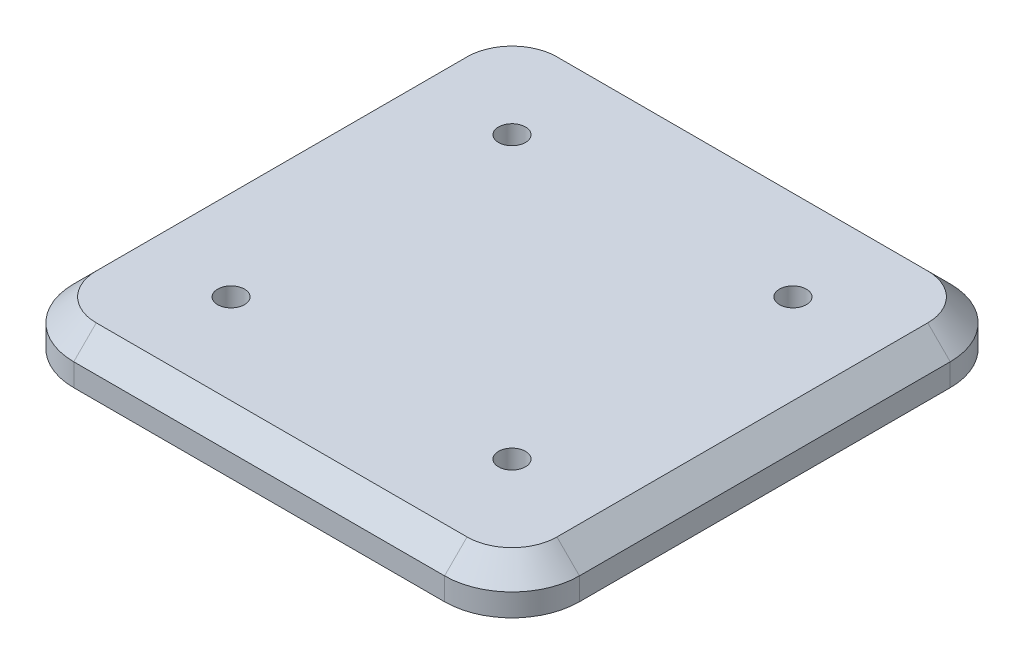
ISO-10303-21;
HEADER;
FILE_DESCRIPTION(('STEP AP214'),'2;1');
FILE_NAME('part.step','',(''),(''),'','','');
FILE_SCHEMA(('AUTOMOTIVE_DESIGN { 1 0 10303 214 1 1 1 1 }'));
ENDSEC;
DATA;
#1=APPLICATION_CONTEXT('core data for automotive mechanical design processes');
#2=APPLICATION_PROTOCOL_DEFINITION('international standard','automotive_design',2000,#1);
#3=PRODUCT_CONTEXT('',#1,'mechanical');
#4=PRODUCT('Part','Part','',(#3));
#5=PRODUCT_RELATED_PRODUCT_CATEGORY('part','',(#4));
#6=PRODUCT_DEFINITION_FORMATION('','',#4);
#7=PRODUCT_DEFINITION_CONTEXT('part definition',#1,'design');
#8=PRODUCT_DEFINITION('design','',#6,#7);
#9=PRODUCT_DEFINITION_SHAPE('','',#8);
#10=(LENGTH_UNIT() NAMED_UNIT(*) SI_UNIT(.MILLI.,.METRE.));
#11=(NAMED_UNIT(*) PLANE_ANGLE_UNIT() SI_UNIT($,.RADIAN.));
#12=(NAMED_UNIT(*) SI_UNIT($,.STERADIAN.) SOLID_ANGLE_UNIT());
#13=UNCERTAINTY_MEASURE_WITH_UNIT(LENGTH_MEASURE(1.E-05),#10,'distance_accuracy_value','');
#14=(GEOMETRIC_REPRESENTATION_CONTEXT(3) GLOBAL_UNCERTAINTY_ASSIGNED_CONTEXT((#13)) GLOBAL_UNIT_ASSIGNED_CONTEXT((#10,
#11,#12)) REPRESENTATION_CONTEXT('',''));
#15=CARTESIAN_POINT('',(0.,0.,0.));
#16=DIRECTION('',(0.,0.,1.));
#17=DIRECTION('',(1.,0.,0.));
#18=AXIS2_PLACEMENT_3D('',#15,#16,#17);
#19=CARTESIAN_POINT('',(112.5,20.,112.5));
#20=DIRECTION('',(-1.,0.,0.));
#21=DIRECTION('',(0.,0.,1.));
#22=AXIS2_PLACEMENT_3D('',#19,#20,#21);
#23=PLANE('',#22);
#24=DIRECTION('',(0.,-1.,0.));
#25=VECTOR('',#24,1.);
#26=CARTESIAN_POINT('',(112.5,20.,-82.5));
#27=LINE('',#26,#25);
#28=CARTESIAN_POINT('',(112.5,0.,-82.5));
#29=VERTEX_POINT('',#28);
#30=CARTESIAN_POINT('',(112.5,9.99999999999996,-82.5));
#31=VERTEX_POINT('',#30);
#32=EDGE_CURVE('E242',#29,#31,#27,.F.);
#33=ORIENTED_EDGE('',*,*,#32,.T.);
#34=DIRECTION('',(0.,0.,1.));
#35=VECTOR('',#34,1.);
#36=CARTESIAN_POINT('',(112.5,9.99999999999996,112.5));
#37=LINE('',#36,#35);
#38=CARTESIAN_POINT('',(112.5,9.99999999999996,82.5));
#39=VERTEX_POINT('',#38);
#40=EDGE_CURVE('E11',#31,#39,#37,.T.);
#41=ORIENTED_EDGE('',*,*,#40,.T.);
#42=DIRECTION('',(0.,-1.,0.));
#43=VECTOR('',#42,1.);
#44=CARTESIAN_POINT('',(112.5,20.,82.5));
#45=LINE('',#44,#43);
#46=CARTESIAN_POINT('',(112.5,0.,82.5));
#47=VERTEX_POINT('',#46);
#48=EDGE_CURVE('E245',#39,#47,#45,.T.);
#49=ORIENTED_EDGE('',*,*,#48,.T.);
#50=DIRECTION('',(0.,0.,-1.));
#51=VECTOR('',#50,1.);
#52=CARTESIAN_POINT('',(112.5,0.,112.5));
#53=LINE('',#52,#51);
#54=EDGE_CURVE('E215',#47,#29,#53,.T.);
#55=ORIENTED_EDGE('',*,*,#54,.T.);
#56=EDGE_LOOP('',(#33,#41,#49,#55));
#57=FACE_BOUND('',#56,.T.);
#58=ADVANCED_FACE('F41',(#57),#23,.F.);
#59=CARTESIAN_POINT('',(-112.5,20.,-112.5));
#60=DIRECTION('',(0.,0.,1.));
#61=DIRECTION('',(1.,0.,0.));
#62=AXIS2_PLACEMENT_3D('',#59,#60,#61);
#63=PLANE('',#62);
#64=DIRECTION('',(0.,-1.,0.));
#65=VECTOR('',#64,1.);
#66=CARTESIAN_POINT('',(-82.5,20.,-112.5));
#67=LINE('',#66,#65);
#68=CARTESIAN_POINT('',(-82.5,0.,-112.5));
#69=VERTEX_POINT('',#68);
#70=CARTESIAN_POINT('',(-82.5,9.99999999999996,-112.5));
#71=VERTEX_POINT('',#70);
#72=EDGE_CURVE('E237',#69,#71,#67,.F.);
#73=ORIENTED_EDGE('',*,*,#72,.T.);
#74=DIRECTION('',(1.,0.,0.));
#75=VECTOR('',#74,1.);
#76=CARTESIAN_POINT('',(-112.5,9.99999999999996,-112.5));
#77=LINE('',#76,#75);
#78=CARTESIAN_POINT('',(82.5,9.99999999999996,-112.5));
#79=VERTEX_POINT('',#78);
#80=EDGE_CURVE('E280',#71,#79,#77,.T.);
#81=ORIENTED_EDGE('',*,*,#80,.T.);
#82=DIRECTION('',(0.,-1.,0.));
#83=VECTOR('',#82,1.);
#84=CARTESIAN_POINT('',(82.5,20.,-112.5));
#85=LINE('',#84,#83);
#86=CARTESIAN_POINT('',(82.5,0.,-112.5));
#87=VERTEX_POINT('',#86);
#88=EDGE_CURVE('E240',#79,#87,#85,.T.);
#89=ORIENTED_EDGE('',*,*,#88,.T.);
#90=DIRECTION('',(-1.,0.,0.));
#91=VECTOR('',#90,1.);
#92=CARTESIAN_POINT('',(-112.5,0.,-112.5));
#93=LINE('',#92,#91);
#94=EDGE_CURVE('E213',#87,#69,#93,.T.);
#95=ORIENTED_EDGE('',*,*,#94,.T.);
#96=EDGE_LOOP('',(#73,#81,#89,#95));
#97=FACE_BOUND('',#96,.T.);
#98=ADVANCED_FACE('F332',(#97),#63,.F.);
#99=CARTESIAN_POINT('',(-112.5,20.,112.5));
#100=DIRECTION('',(1.,0.,0.));
#101=DIRECTION('',(0.,0.,-1.));
#102=AXIS2_PLACEMENT_3D('',#99,#100,#101);
#103=PLANE('',#102);
#104=DIRECTION('',(0.,-1.,0.));
#105=VECTOR('',#104,1.);
#106=CARTESIAN_POINT('',(-112.5,20.,82.5));
#107=LINE('',#106,#105);
#108=CARTESIAN_POINT('',(-112.5,0.,82.5));
#109=VERTEX_POINT('',#108);
#110=CARTESIAN_POINT('',(-112.5,9.99999999999996,82.5));
#111=VERTEX_POINT('',#110);
#112=EDGE_CURVE('E223',#109,#111,#107,.F.);
#113=ORIENTED_EDGE('',*,*,#112,.T.);
#114=DIRECTION('',(0.,0.,-1.));
#115=VECTOR('',#114,1.);
#116=CARTESIAN_POINT('',(-112.5,9.99999999999996,112.5));
#117=LINE('',#116,#115);
#118=CARTESIAN_POINT('',(-112.5,9.99999999999996,-82.5));
#119=VERTEX_POINT('',#118);
#120=EDGE_CURVE('E269',#111,#119,#117,.T.);
#121=ORIENTED_EDGE('',*,*,#120,.T.);
#122=DIRECTION('',(0.,-1.,0.));
#123=VECTOR('',#122,1.);
#124=CARTESIAN_POINT('',(-112.5,20.,-82.5));
#125=LINE('',#124,#123);
#126=CARTESIAN_POINT('',(-112.5,0.,-82.5));
#127=VERTEX_POINT('',#126);
#128=EDGE_CURVE('E227',#119,#127,#125,.T.);
#129=ORIENTED_EDGE('',*,*,#128,.T.);
#130=DIRECTION('',(0.,0.,1.));
#131=VECTOR('',#130,1.);
#132=CARTESIAN_POINT('',(-112.5,0.,112.5));
#133=LINE('',#132,#131);
#134=EDGE_CURVE('E220',#127,#109,#133,.T.);
#135=ORIENTED_EDGE('',*,*,#134,.T.);
#136=EDGE_LOOP('',(#113,#121,#129,#135));
#137=FACE_BOUND('',#136,.T.);
#138=ADVANCED_FACE('F349',(#137),#103,.F.);
#139=CARTESIAN_POINT('',(-112.5,20.,112.5));
#140=DIRECTION('',(0.,0.,-1.));
#141=DIRECTION('',(-1.,0.,0.));
#142=AXIS2_PLACEMENT_3D('',#139,#140,#141);
#143=PLANE('',#142);
#144=DIRECTION('',(0.,-1.,0.));
#145=VECTOR('',#144,1.);
#146=CARTESIAN_POINT('',(82.5,20.,112.5));
#147=LINE('',#146,#145);
#148=CARTESIAN_POINT('',(82.5,0.,112.5));
#149=VERTEX_POINT('',#148);
#150=CARTESIAN_POINT('',(82.5,9.99999999999996,112.5));
#151=VERTEX_POINT('',#150);
#152=EDGE_CURVE('E247',#149,#151,#147,.F.);
#153=ORIENTED_EDGE('',*,*,#152,.T.);
#154=DIRECTION('',(-1.,0.,0.));
#155=VECTOR('',#154,1.);
#156=CARTESIAN_POINT('',(-112.5,9.99999999999996,112.5));
#157=LINE('',#156,#155);
#158=CARTESIAN_POINT('',(-82.5,9.99999999999996,112.5));
#159=VERTEX_POINT('',#158);
#160=EDGE_CURVE('E273',#151,#159,#157,.T.);
#161=ORIENTED_EDGE('',*,*,#160,.T.);
#162=DIRECTION('',(0.,-1.,0.));
#163=VECTOR('',#162,1.);
#164=CARTESIAN_POINT('',(-82.5,20.,112.5));
#165=LINE('',#164,#163);
#166=CARTESIAN_POINT('',(-82.5,0.,112.5));
#167=VERTEX_POINT('',#166);
#168=EDGE_CURVE('E246',#159,#167,#165,.T.);
#169=ORIENTED_EDGE('',*,*,#168,.T.);
#170=DIRECTION('',(1.,0.,0.));
#171=VECTOR('',#170,1.);
#172=CARTESIAN_POINT('',(-112.5,0.,112.5));
#173=LINE('',#172,#171);
#174=EDGE_CURVE('E221',#167,#149,#173,.T.);
#175=ORIENTED_EDGE('',*,*,#174,.T.);
#176=EDGE_LOOP('',(#153,#161,#169,#175));
#177=FACE_BOUND('',#176,.T.);
#178=ADVANCED_FACE('F319',(#177),#143,.F.);
#179=CARTESIAN_POINT('',(0.,20.,0.));
#180=DIRECTION('',(0.,-1.,0.));
#181=DIRECTION('',(0.,0.,-1.));
#182=AXIS2_PLACEMENT_3D('',#179,#180,#181);
#183=PLANE('',#182);
#184=CARTESIAN_POINT('',(62.5,20.,62.5));
#185=DIRECTION('',(0.,1.,0.));
#186=DIRECTION('',(0.,0.,1.));
#187=AXIS2_PLACEMENT_3D('',#184,#185,#186);
#188=CIRCLE('',#187,5.99999999999998);
#189=CARTESIAN_POINT('',(62.5,20.,68.5));
#190=VERTEX_POINT('',#189);
#191=EDGE_CURVE('E190',#190,#190,#188,.T.);
#192=ORIENTED_EDGE('',*,*,#191,.F.);
#193=EDGE_LOOP('',(#192));
#194=FACE_BOUND('',#193,.T.);
#195=CARTESIAN_POINT('',(-62.5,20.,62.5));
#196=DIRECTION('',(0.,1.,0.));
#197=DIRECTION('',(0.,0.,1.));
#198=AXIS2_PLACEMENT_3D('',#195,#196,#197);
#199=CIRCLE('',#198,5.99999999999999);
#200=CARTESIAN_POINT('',(-62.5,20.,68.5));
#201=VERTEX_POINT('',#200);
#202=EDGE_CURVE('E194',#201,#201,#199,.T.);
#203=ORIENTED_EDGE('',*,*,#202,.F.);
#204=EDGE_LOOP('',(#203));
#205=FACE_BOUND('',#204,.T.);
#206=CARTESIAN_POINT('',(-62.5,20.,-62.5));
#207=DIRECTION('',(0.,1.,0.));
#208=DIRECTION('',(0.,0.,1.));
#209=AXIS2_PLACEMENT_3D('',#206,#207,#208);
#210=CIRCLE('',#209,5.99999999999999);
#211=CARTESIAN_POINT('',(-62.5,20.,-56.5));
#212=VERTEX_POINT('',#211);
#213=EDGE_CURVE('E198',#212,#212,#210,.T.);
#214=ORIENTED_EDGE('',*,*,#213,.F.);
#215=EDGE_LOOP('',(#214));
#216=FACE_BOUND('',#215,.T.);
#217=CARTESIAN_POINT('',(62.5,20.,-62.5));
#218=DIRECTION('',(0.,1.,0.));
#219=DIRECTION('',(0.,0.,1.));
#220=AXIS2_PLACEMENT_3D('',#217,#218,#219);
#221=CIRCLE('',#220,5.99999999999998);
#222=CARTESIAN_POINT('',(62.5,20.,-56.5));
#223=VERTEX_POINT('',#222);
#224=EDGE_CURVE('E205',#223,#223,#221,.T.);
#225=ORIENTED_EDGE('',*,*,#224,.F.);
#226=EDGE_LOOP('',(#225));
#227=FACE_BOUND('',#226,.T.);
#228=CARTESIAN_POINT('',(-82.5,20.,-82.5));
#229=DIRECTION('',(0.,-1.,0.));
#230=DIRECTION('',(0.,0.,-1.));
#231=AXIS2_PLACEMENT_3D('',#228,#229,#230);
#232=CIRCLE('',#231,20.);
#233=CARTESIAN_POINT('',(-82.5,20.,-102.5));
#234=VERTEX_POINT('',#233);
#235=CARTESIAN_POINT('',(-102.5,20.,-82.5));
#236=VERTEX_POINT('',#235);
#237=EDGE_CURVE('E264',#234,#236,#232,.F.);
#238=ORIENTED_EDGE('',*,*,#237,.T.);
#239=DIRECTION('',(0.,0.,1.));
#240=VECTOR('',#239,1.);
#241=CARTESIAN_POINT('',(-102.5,20.,0.));
#242=LINE('',#241,#240);
#243=CARTESIAN_POINT('',(-102.5,20.,82.5));
#244=VERTEX_POINT('',#243);
#245=EDGE_CURVE('E262',#236,#244,#242,.T.);
#246=ORIENTED_EDGE('',*,*,#245,.T.);
#247=CARTESIAN_POINT('',(-82.5,20.,82.5));
#248=DIRECTION('',(0.,-1.,0.));
#249=DIRECTION('',(0.,0.,-1.));
#250=AXIS2_PLACEMENT_3D('',#247,#248,#249);
#251=CIRCLE('',#250,20.);
#252=CARTESIAN_POINT('',(-82.5,20.,102.5));
#253=VERTEX_POINT('',#252);
#254=EDGE_CURVE('E265',#244,#253,#251,.F.);
#255=ORIENTED_EDGE('',*,*,#254,.T.);
#256=DIRECTION('',(1.,0.,0.));
#257=VECTOR('',#256,1.);
#258=CARTESIAN_POINT('',(0.,20.,102.5));
#259=LINE('',#258,#257);
#260=CARTESIAN_POINT('',(82.5,20.,102.5));
#261=VERTEX_POINT('',#260);
#262=EDGE_CURVE('E256',#253,#261,#259,.T.);
#263=ORIENTED_EDGE('',*,*,#262,.T.);
#264=CARTESIAN_POINT('',(82.5,20.,82.5));
#265=DIRECTION('',(0.,-1.,0.));
#266=DIRECTION('',(0.,0.,-1.));
#267=AXIS2_PLACEMENT_3D('',#264,#265,#266);
#268=CIRCLE('',#267,20.);
#269=CARTESIAN_POINT('',(102.5,20.,82.5));
#270=VERTEX_POINT('',#269);
#271=EDGE_CURVE('E253',#261,#270,#268,.F.);
#272=ORIENTED_EDGE('',*,*,#271,.T.);
#273=DIRECTION('',(0.,0.,-1.));
#274=VECTOR('',#273,1.);
#275=CARTESIAN_POINT('',(102.5,20.,0.));
#276=LINE('',#275,#274);
#277=CARTESIAN_POINT('',(102.5,20.,-82.5));
#278=VERTEX_POINT('',#277);
#279=EDGE_CURVE('E252',#270,#278,#276,.T.);
#280=ORIENTED_EDGE('',*,*,#279,.T.);
#281=CARTESIAN_POINT('',(82.5,20.,-82.5));
#282=DIRECTION('',(0.,-1.,0.));
#283=DIRECTION('',(0.,0.,-1.));
#284=AXIS2_PLACEMENT_3D('',#281,#282,#283);
#285=CIRCLE('',#284,20.);
#286=CARTESIAN_POINT('',(82.5,20.,-102.5));
#287=VERTEX_POINT('',#286);
#288=EDGE_CURVE('E254',#278,#287,#285,.F.);
#289=ORIENTED_EDGE('',*,*,#288,.T.);
#290=DIRECTION('',(-1.,0.,0.));
#291=VECTOR('',#290,1.);
#292=CARTESIAN_POINT('',(0.,20.,-102.5));
#293=LINE('',#292,#291);
#294=EDGE_CURVE('E260',#287,#234,#293,.T.);
#295=ORIENTED_EDGE('',*,*,#294,.T.);
#296=EDGE_LOOP('',(#238,#246,#255,#263,#272,#280,#289,#295));
#297=FACE_BOUND('',#296,.T.);
#298=ADVANCED_FACE('F356',(#194,#205,#216,#227,#297),#183,.F.);
#299=CARTESIAN_POINT('',(0.,0.,0.));
#300=DIRECTION('',(0.,-1.,0.));
#301=DIRECTION('',(0.,0.,-1.));
#302=AXIS2_PLACEMENT_3D('',#299,#300,#301);
#303=PLANE('',#302);
#304=CARTESIAN_POINT('',(-87.5,0.,87.5));
#305=DIRECTION('',(0.,-1.,0.));
#306=DIRECTION('',(0.,0.,-1.));
#307=AXIS2_PLACEMENT_3D('',#304,#305,#306);
#308=CIRCLE('',#307,5.99999999999999);
#309=CARTESIAN_POINT('',(-87.5,0.,81.5));
#310=VERTEX_POINT('',#309);
#311=EDGE_CURVE('E164',#310,#310,#308,.T.);
#312=ORIENTED_EDGE('',*,*,#311,.F.);
#313=EDGE_LOOP('',(#312));
#314=FACE_BOUND('',#313,.T.);
#315=CARTESIAN_POINT('',(87.5,0.,87.5));
#316=DIRECTION('',(0.,-1.,0.));
#317=DIRECTION('',(0.,0.,-1.));
#318=AXIS2_PLACEMENT_3D('',#315,#316,#317);
#319=CIRCLE('',#318,5.99999999999999);
#320=CARTESIAN_POINT('',(87.5,0.,81.5));
#321=VERTEX_POINT('',#320);
#322=EDGE_CURVE('E165',#321,#321,#319,.T.);
#323=ORIENTED_EDGE('',*,*,#322,.F.);
#324=EDGE_LOOP('',(#323));
#325=FACE_BOUND('',#324,.T.);
#326=CARTESIAN_POINT('',(87.5,0.,-87.5));
#327=DIRECTION('',(0.,-1.,0.));
#328=DIRECTION('',(0.,0.,-1.));
#329=AXIS2_PLACEMENT_3D('',#326,#327,#328);
#330=CIRCLE('',#329,5.99999999999999);
#331=CARTESIAN_POINT('',(87.5,0.,-93.5));
#332=VERTEX_POINT('',#331);
#333=EDGE_CURVE('E174',#332,#332,#330,.T.);
#334=ORIENTED_EDGE('',*,*,#333,.F.);
#335=EDGE_LOOP('',(#334));
#336=FACE_BOUND('',#335,.T.);
#337=CARTESIAN_POINT('',(-87.5,0.,-87.5));
#338=DIRECTION('',(0.,-1.,0.));
#339=DIRECTION('',(0.,0.,-1.));
#340=AXIS2_PLACEMENT_3D('',#337,#338,#339);
#341=CIRCLE('',#340,5.99999999999999);
#342=CARTESIAN_POINT('',(-87.5,0.,-93.5));
#343=VERTEX_POINT('',#342);
#344=EDGE_CURVE('E181',#343,#343,#341,.T.);
#345=ORIENTED_EDGE('',*,*,#344,.F.);
#346=EDGE_LOOP('',(#345));
#347=FACE_BOUND('',#346,.T.);
#348=ORIENTED_EDGE('',*,*,#134,.F.);
#349=CARTESIAN_POINT('',(-82.5,0.,-82.5));
#350=DIRECTION('',(0.,-1.,0.));
#351=DIRECTION('',(0.,0.,-1.));
#352=AXIS2_PLACEMENT_3D('',#349,#350,#351);
#353=CIRCLE('',#352,30.);
#354=EDGE_CURVE('E232',#127,#69,#353,.T.);
#355=ORIENTED_EDGE('',*,*,#354,.T.);
#356=ORIENTED_EDGE('',*,*,#94,.F.);
#357=CARTESIAN_POINT('',(82.5,0.,-82.5));
#358=DIRECTION('',(0.,-1.,0.));
#359=DIRECTION('',(0.,0.,-1.));
#360=AXIS2_PLACEMENT_3D('',#357,#358,#359);
#361=CIRCLE('',#360,30.);
#362=EDGE_CURVE('E231',#87,#29,#361,.T.);
#363=ORIENTED_EDGE('',*,*,#362,.T.);
#364=ORIENTED_EDGE('',*,*,#54,.F.);
#365=CARTESIAN_POINT('',(82.5,0.,82.5));
#366=DIRECTION('',(0.,-1.,0.));
#367=DIRECTION('',(0.,0.,-1.));
#368=AXIS2_PLACEMENT_3D('',#365,#366,#367);
#369=CIRCLE('',#368,30.);
#370=EDGE_CURVE('E233',#47,#149,#369,.T.);
#371=ORIENTED_EDGE('',*,*,#370,.T.);
#372=ORIENTED_EDGE('',*,*,#174,.F.);
#373=CARTESIAN_POINT('',(-82.5,0.,82.5));
#374=DIRECTION('',(0.,-1.,0.));
#375=DIRECTION('',(0.,0.,-1.));
#376=AXIS2_PLACEMENT_3D('',#373,#374,#375);
#377=CIRCLE('',#376,30.);
#378=EDGE_CURVE('E230',#167,#109,#377,.T.);
#379=ORIENTED_EDGE('',*,*,#378,.T.);
#380=EDGE_LOOP('',(#348,#355,#356,#363,#364,#371,#372,#379));
#381=FACE_BOUND('',#380,.T.);
#382=ADVANCED_FACE('F321',(#314,#325,#336,#347,#381),#303,.T.);
#383=CARTESIAN_POINT('',(-82.5,20.,-82.5));
#384=DIRECTION('',(0.,-1.,0.));
#385=DIRECTION('',(0.,0.,-1.));
#386=AXIS2_PLACEMENT_3D('',#383,#384,#385);
#387=CYLINDRICAL_SURFACE('',#386,30.);
#388=ORIENTED_EDGE('',*,*,#128,.F.);
#389=CARTESIAN_POINT('',(-82.5,9.99999999999996,-82.5));
#390=DIRECTION('',(0.,-1.,0.));
#391=DIRECTION('',(0.,0.,-1.));
#392=AXIS2_PLACEMENT_3D('',#389,#390,#391);
#393=CIRCLE('',#392,30.);
#394=EDGE_CURVE('E271',#119,#71,#393,.T.);
#395=ORIENTED_EDGE('',*,*,#394,.T.);
#396=ORIENTED_EDGE('',*,*,#72,.F.);
#397=ORIENTED_EDGE('',*,*,#354,.F.);
#398=EDGE_LOOP('',(#388,#395,#396,#397));
#399=FACE_BOUND('',#398,.T.);
#400=ADVANCED_FACE('F337',(#399),#387,.T.);
#401=CARTESIAN_POINT('',(82.5,20.,-82.5));
#402=DIRECTION('',(0.,-1.,0.));
#403=DIRECTION('',(0.,0.,-1.));
#404=AXIS2_PLACEMENT_3D('',#401,#402,#403);
#405=CYLINDRICAL_SURFACE('',#404,30.);
#406=ORIENTED_EDGE('',*,*,#88,.F.);
#407=CARTESIAN_POINT('',(82.5,9.99999999999996,-82.5));
#408=DIRECTION('',(0.,-1.,0.));
#409=DIRECTION('',(0.,0.,-1.));
#410=AXIS2_PLACEMENT_3D('',#407,#408,#409);
#411=CIRCLE('',#410,30.);
#412=EDGE_CURVE('E51',#79,#31,#411,.T.);
#413=ORIENTED_EDGE('',*,*,#412,.T.);
#414=ORIENTED_EDGE('',*,*,#32,.F.);
#415=ORIENTED_EDGE('',*,*,#362,.F.);
#416=EDGE_LOOP('',(#406,#413,#414,#415));
#417=FACE_BOUND('',#416,.T.);
#418=ADVANCED_FACE('F330',(#417),#405,.T.);
#419=CARTESIAN_POINT('',(82.5,20.,82.5));
#420=DIRECTION('',(0.,-1.,0.));
#421=DIRECTION('',(0.,0.,-1.));
#422=AXIS2_PLACEMENT_3D('',#419,#420,#421);
#423=CYLINDRICAL_SURFACE('',#422,30.);
#424=ORIENTED_EDGE('',*,*,#48,.F.);
#425=CARTESIAN_POINT('',(82.5,9.99999999999996,82.5));
#426=DIRECTION('',(0.,-1.,0.));
#427=DIRECTION('',(0.,0.,-1.));
#428=AXIS2_PLACEMENT_3D('',#425,#426,#427);
#429=CIRCLE('',#428,30.);
#430=EDGE_CURVE('E276',#39,#151,#429,.T.);
#431=ORIENTED_EDGE('',*,*,#430,.T.);
#432=ORIENTED_EDGE('',*,*,#152,.F.);
#433=ORIENTED_EDGE('',*,*,#370,.F.);
#434=EDGE_LOOP('',(#424,#431,#432,#433));
#435=FACE_BOUND('',#434,.T.);
#436=ADVANCED_FACE('F314',(#435),#423,.T.);
#437=CARTESIAN_POINT('',(-82.5,20.,82.5));
#438=DIRECTION('',(0.,-1.,0.));
#439=DIRECTION('',(0.,0.,-1.));
#440=AXIS2_PLACEMENT_3D('',#437,#438,#439);
#441=CYLINDRICAL_SURFACE('',#440,30.);
#442=ORIENTED_EDGE('',*,*,#168,.F.);
#443=CARTESIAN_POINT('',(-82.5,9.99999999999996,82.5));
#444=DIRECTION('',(0.,-1.,0.));
#445=DIRECTION('',(0.,0.,-1.));
#446=AXIS2_PLACEMENT_3D('',#443,#444,#445);
#447=CIRCLE('',#446,30.);
#448=EDGE_CURVE('E272',#159,#111,#447,.T.);
#449=ORIENTED_EDGE('',*,*,#448,.T.);
#450=ORIENTED_EDGE('',*,*,#112,.F.);
#451=ORIENTED_EDGE('',*,*,#378,.F.);
#452=EDGE_LOOP('',(#442,#449,#450,#451));
#453=FACE_BOUND('',#452,.T.);
#454=ADVANCED_FACE('F390',(#453),#441,.T.);
#455=CARTESIAN_POINT('',(102.5,20.,0.));
#456=DIRECTION('',(-0.707106781186549,-0.707106781186545,0.));
#457=DIRECTION('',(0.,0.,-1.));
#458=AXIS2_PLACEMENT_3D('',#455,#456,#457);
#459=PLANE('',#458);
#460=DIRECTION('',(-0.707106781186545,0.70710678118655,0.));
#461=VECTOR('',#460,1.);
#462=CARTESIAN_POINT('',(112.5,9.99999999999996,82.5));
#463=LINE('',#462,#461);
#464=EDGE_CURVE('E298',#39,#270,#463,.T.);
#465=ORIENTED_EDGE('',*,*,#464,.F.);
#466=ORIENTED_EDGE('',*,*,#40,.F.);
#467=DIRECTION('',(0.707106781186545,-0.70710678118655,0.));
#468=VECTOR('',#467,1.);
#469=CARTESIAN_POINT('',(102.5,20.,-82.5));
#470=LINE('',#469,#468);
#471=EDGE_CURVE('E46',#278,#31,#470,.T.);
#472=ORIENTED_EDGE('',*,*,#471,.F.);
#473=ORIENTED_EDGE('',*,*,#279,.F.);
#474=EDGE_LOOP('',(#465,#466,#472,#473));
#475=FACE_BOUND('',#474,.T.);
#476=ADVANCED_FACE('F42',(#475),#459,.F.);
#477=CARTESIAN_POINT('',(82.5,20.,-82.5));
#478=DIRECTION('',(0.,-1.,0.));
#479=DIRECTION('',(0.,0.,-1.));
#480=AXIS2_PLACEMENT_3D('',#477,#478,#479);
#481=CONICAL_SURFACE('',#480,20.,0.785398163397446);
#482=ORIENTED_EDGE('',*,*,#471,.T.);
#483=ORIENTED_EDGE('',*,*,#412,.F.);
#484=DIRECTION('',(0.,-0.707106781186549,-0.707106781186545));
#485=VECTOR('',#484,1.);
#486=CARTESIAN_POINT('',(82.5,20.,-102.5));
#487=LINE('',#486,#485);
#488=EDGE_CURVE('E295',#287,#79,#487,.T.);
#489=ORIENTED_EDGE('',*,*,#488,.F.);
#490=ORIENTED_EDGE('',*,*,#288,.F.);
#491=EDGE_LOOP('',(#482,#483,#489,#490));
#492=FACE_BOUND('',#491,.T.);
#493=ADVANCED_FACE('F306',(#492),#481,.T.);
#494=CARTESIAN_POINT('',(82.5,20.,82.5));
#495=DIRECTION('',(0.,-1.,0.));
#496=DIRECTION('',(0.,0.,-1.));
#497=AXIS2_PLACEMENT_3D('',#494,#495,#496);
#498=CONICAL_SURFACE('',#497,20.,0.785398163397446);
#499=ORIENTED_EDGE('',*,*,#464,.T.);
#500=ORIENTED_EDGE('',*,*,#271,.F.);
#501=DIRECTION('',(0.,0.707106781186549,-0.707106781186545));
#502=VECTOR('',#501,1.);
#503=CARTESIAN_POINT('',(82.5,9.99999999999996,112.5));
#504=LINE('',#503,#502);
#505=EDGE_CURVE('E293',#151,#261,#504,.T.);
#506=ORIENTED_EDGE('',*,*,#505,.F.);
#507=ORIENTED_EDGE('',*,*,#430,.F.);
#508=EDGE_LOOP('',(#499,#500,#506,#507));
#509=FACE_BOUND('',#508,.T.);
#510=ADVANCED_FACE('F311',(#509),#498,.T.);
#511=CARTESIAN_POINT('',(0.,20.,-102.5));
#512=DIRECTION('',(0.,-0.707106781186545,0.707106781186549));
#513=DIRECTION('',(-1.,0.,0.));
#514=AXIS2_PLACEMENT_3D('',#511,#512,#513);
#515=PLANE('',#514);
#516=ORIENTED_EDGE('',*,*,#488,.T.);
#517=ORIENTED_EDGE('',*,*,#80,.F.);
#518=DIRECTION('',(0.,-0.70710678118655,-0.707106781186545));
#519=VECTOR('',#518,1.);
#520=CARTESIAN_POINT('',(-82.5,20.,-102.5));
#521=LINE('',#520,#519);
#522=EDGE_CURVE('E289',#234,#71,#521,.T.);
#523=ORIENTED_EDGE('',*,*,#522,.F.);
#524=ORIENTED_EDGE('',*,*,#294,.F.);
#525=EDGE_LOOP('',(#516,#517,#523,#524));
#526=FACE_BOUND('',#525,.T.);
#527=ADVANCED_FACE('F363',(#526),#515,.F.);
#528=CARTESIAN_POINT('',(0.,20.,102.5));
#529=DIRECTION('',(0.,-0.707106781186545,-0.707106781186549));
#530=DIRECTION('',(1.,0.,0.));
#531=AXIS2_PLACEMENT_3D('',#528,#529,#530);
#532=PLANE('',#531);
#533=ORIENTED_EDGE('',*,*,#505,.T.);
#534=ORIENTED_EDGE('',*,*,#262,.F.);
#535=DIRECTION('',(0.,0.70710678118655,-0.707106781186545));
#536=VECTOR('',#535,1.);
#537=CARTESIAN_POINT('',(-82.5,9.99999999999996,112.5));
#538=LINE('',#537,#536);
#539=EDGE_CURVE('E282',#159,#253,#538,.T.);
#540=ORIENTED_EDGE('',*,*,#539,.F.);
#541=ORIENTED_EDGE('',*,*,#160,.F.);
#542=EDGE_LOOP('',(#533,#534,#540,#541));
#543=FACE_BOUND('',#542,.T.);
#544=ADVANCED_FACE('F361',(#543),#532,.F.);
#545=CARTESIAN_POINT('',(-82.5,20.,-82.5));
#546=DIRECTION('',(0.,-1.,0.));
#547=DIRECTION('',(0.,0.,-1.));
#548=AXIS2_PLACEMENT_3D('',#545,#546,#547);
#549=CONICAL_SURFACE('',#548,20.,0.785398163397446);
#550=ORIENTED_EDGE('',*,*,#522,.T.);
#551=ORIENTED_EDGE('',*,*,#394,.F.);
#552=DIRECTION('',(-0.707106781186545,-0.707106781186549,0.));
#553=VECTOR('',#552,1.);
#554=CARTESIAN_POINT('',(-102.5,20.,-82.5));
#555=LINE('',#554,#553);
#556=EDGE_CURVE('E285',#236,#119,#555,.T.);
#557=ORIENTED_EDGE('',*,*,#556,.F.);
#558=ORIENTED_EDGE('',*,*,#237,.F.);
#559=EDGE_LOOP('',(#550,#551,#557,#558));
#560=FACE_BOUND('',#559,.T.);
#561=ADVANCED_FACE('F338',(#560),#549,.T.);
#562=CARTESIAN_POINT('',(-82.5,20.,82.5));
#563=DIRECTION('',(0.,-1.,0.));
#564=DIRECTION('',(0.,0.,-1.));
#565=AXIS2_PLACEMENT_3D('',#562,#563,#564);
#566=CONICAL_SURFACE('',#565,20.,0.785398163397446);
#567=ORIENTED_EDGE('',*,*,#539,.T.);
#568=ORIENTED_EDGE('',*,*,#254,.F.);
#569=DIRECTION('',(0.707106781186545,0.707106781186549,0.));
#570=VECTOR('',#569,1.);
#571=CARTESIAN_POINT('',(-112.5,9.99999999999996,82.5));
#572=LINE('',#571,#570);
#573=EDGE_CURVE('E212',#111,#244,#572,.T.);
#574=ORIENTED_EDGE('',*,*,#573,.F.);
#575=ORIENTED_EDGE('',*,*,#448,.F.);
#576=EDGE_LOOP('',(#567,#568,#574,#575));
#577=FACE_BOUND('',#576,.T.);
#578=ADVANCED_FACE('F353',(#577),#566,.T.);
#579=CARTESIAN_POINT('',(-102.5,20.,0.));
#580=DIRECTION('',(0.707106781186549,-0.707106781186545,0.));
#581=DIRECTION('',(0.,0.,1.));
#582=AXIS2_PLACEMENT_3D('',#579,#580,#581);
#583=PLANE('',#582);
#584=ORIENTED_EDGE('',*,*,#556,.T.);
#585=ORIENTED_EDGE('',*,*,#120,.F.);
#586=ORIENTED_EDGE('',*,*,#573,.T.);
#587=ORIENTED_EDGE('',*,*,#245,.F.);
#588=EDGE_LOOP('',(#584,#585,#586,#587));
#589=FACE_BOUND('',#588,.T.);
#590=ADVANCED_FACE('F347',(#589),#583,.F.);
#591=CARTESIAN_POINT('',(62.5,10.,-62.5));
#592=DIRECTION('',(0.,1.,0.));
#593=DIRECTION('',(0.,0.,1.));
#594=AXIS2_PLACEMENT_3D('',#591,#592,#593);
#595=CONICAL_SURFACE('',#594,5.99999999999998,1.02974425867665);
#596=CARTESIAN_POINT('',(62.5,6.39483628583465,-62.5));
#597=VERTEX_POINT('',#596);
#598=VERTEX_LOOP('',#597);
#599=FACE_BOUND('',#598,.T.);
#600=CARTESIAN_POINT('',(62.5,10.,-62.5));
#601=DIRECTION('',(0.,1.,0.));
#602=DIRECTION('',(0.,0.,1.));
#603=AXIS2_PLACEMENT_3D('',#600,#601,#602);
#604=CIRCLE('',#603,5.99999999999998);
#605=CARTESIAN_POINT('',(62.5,10.,-56.5));
#606=VERTEX_POINT('',#605);
#607=EDGE_CURVE('E206',#606,#606,#604,.T.);
#608=ORIENTED_EDGE('',*,*,#607,.T.);
#609=EDGE_LOOP('',(#608));
#610=FACE_BOUND('',#609,.T.);
#611=ADVANCED_FACE('F397',(#599,#610),#595,.F.);
#612=CARTESIAN_POINT('',(62.5,20.,-62.5));
#613=DIRECTION('',(0.,1.,0.));
#614=DIRECTION('',(0.,0.,1.));
#615=AXIS2_PLACEMENT_3D('',#612,#613,#614);
#616=CYLINDRICAL_SURFACE('',#615,5.99999999999998);
#617=ORIENTED_EDGE('',*,*,#607,.F.);
#618=EDGE_LOOP('',(#617));
#619=FACE_BOUND('',#618,.T.);
#620=ORIENTED_EDGE('',*,*,#224,.T.);
#621=EDGE_LOOP('',(#620));
#622=FACE_BOUND('',#621,.T.);
#623=ADVANCED_FACE('F535',(#619,#622),#616,.F.);
#624=CARTESIAN_POINT('',(-62.5,10.,-62.5));
#625=DIRECTION('',(0.,1.,0.));
#626=DIRECTION('',(0.,0.,1.));
#627=AXIS2_PLACEMENT_3D('',#624,#625,#626);
#628=CONICAL_SURFACE('',#627,5.99999999999998,1.02974425867665);
#629=CARTESIAN_POINT('',(-62.5,6.39483628583465,-62.5));
#630=VERTEX_POINT('',#629);
#631=VERTEX_LOOP('',#630);
#632=FACE_BOUND('',#631,.T.);
#633=CARTESIAN_POINT('',(-62.5,10.,-62.5));
#634=DIRECTION('',(0.,1.,0.));
#635=DIRECTION('',(0.,0.,1.));
#636=AXIS2_PLACEMENT_3D('',#633,#634,#635);
#637=CIRCLE('',#636,5.99999999999998);
#638=CARTESIAN_POINT('',(-62.5,10.,-56.5));
#639=VERTEX_POINT('',#638);
#640=EDGE_CURVE('E202',#639,#639,#637,.T.);
#641=ORIENTED_EDGE('',*,*,#640,.T.);
#642=EDGE_LOOP('',(#641));
#643=FACE_BOUND('',#642,.T.);
#644=ADVANCED_FACE('F544',(#632,#643),#628,.F.);
#645=CARTESIAN_POINT('',(-62.5,20.,-62.5));
#646=DIRECTION('',(0.,1.,0.));
#647=DIRECTION('',(0.,0.,1.));
#648=AXIS2_PLACEMENT_3D('',#645,#646,#647);
#649=CYLINDRICAL_SURFACE('',#648,5.99999999999999);
#650=ORIENTED_EDGE('',*,*,#640,.F.);
#651=EDGE_LOOP('',(#650));
#652=FACE_BOUND('',#651,.T.);
#653=ORIENTED_EDGE('',*,*,#213,.T.);
#654=EDGE_LOOP('',(#653));
#655=FACE_BOUND('',#654,.T.);
#656=ADVANCED_FACE('F550',(#652,#655),#649,.F.);
#657=CARTESIAN_POINT('',(-62.5,10.,62.5));
#658=DIRECTION('',(0.,1.,0.));
#659=DIRECTION('',(0.,0.,1.));
#660=AXIS2_PLACEMENT_3D('',#657,#658,#659);
#661=CONICAL_SURFACE('',#660,5.99999999999998,1.02974425867665);
#662=CARTESIAN_POINT('',(-62.5,6.39483628583465,62.5));
#663=VERTEX_POINT('',#662);
#664=VERTEX_LOOP('',#663);
#665=FACE_BOUND('',#664,.T.);
#666=CARTESIAN_POINT('',(-62.5,10.,62.5));
#667=DIRECTION('',(0.,1.,0.));
#668=DIRECTION('',(0.,0.,1.));
#669=AXIS2_PLACEMENT_3D('',#666,#667,#668);
#670=CIRCLE('',#669,5.99999999999998);
#671=CARTESIAN_POINT('',(-62.5,10.,68.5));
#672=VERTEX_POINT('',#671);
#673=EDGE_CURVE('E199',#672,#672,#670,.T.);
#674=ORIENTED_EDGE('',*,*,#673,.T.);
#675=EDGE_LOOP('',(#674));
#676=FACE_BOUND('',#675,.T.);
#677=ADVANCED_FACE('F559',(#665,#676),#661,.F.);
#678=CARTESIAN_POINT('',(-62.5,20.,62.5));
#679=DIRECTION('',(0.,1.,0.));
#680=DIRECTION('',(0.,0.,1.));
#681=AXIS2_PLACEMENT_3D('',#678,#679,#680);
#682=CYLINDRICAL_SURFACE('',#681,5.99999999999999);
#683=ORIENTED_EDGE('',*,*,#673,.F.);
#684=EDGE_LOOP('',(#683));
#685=FACE_BOUND('',#684,.T.);
#686=ORIENTED_EDGE('',*,*,#202,.T.);
#687=EDGE_LOOP('',(#686));
#688=FACE_BOUND('',#687,.T.);
#689=ADVANCED_FACE('F568',(#685,#688),#682,.F.);
#690=CARTESIAN_POINT('',(62.5,10.,62.5));
#691=DIRECTION('',(0.,1.,0.));
#692=DIRECTION('',(0.,0.,1.));
#693=AXIS2_PLACEMENT_3D('',#690,#691,#692);
#694=CONICAL_SURFACE('',#693,5.99999999999998,1.02974425867665);
#695=CARTESIAN_POINT('',(62.5,6.39483628583465,62.5));
#696=VERTEX_POINT('',#695);
#697=VERTEX_LOOP('',#696);
#698=FACE_BOUND('',#697,.T.);
#699=CARTESIAN_POINT('',(62.5,10.,62.5));
#700=DIRECTION('',(0.,1.,0.));
#701=DIRECTION('',(0.,0.,1.));
#702=AXIS2_PLACEMENT_3D('',#699,#700,#701);
#703=CIRCLE('',#702,5.99999999999998);
#704=CARTESIAN_POINT('',(62.5,10.,68.5));
#705=VERTEX_POINT('',#704);
#706=EDGE_CURVE('E188',#705,#705,#703,.T.);
#707=ORIENTED_EDGE('',*,*,#706,.T.);
#708=EDGE_LOOP('',(#707));
#709=FACE_BOUND('',#708,.T.);
#710=ADVANCED_FACE('F580',(#698,#709),#694,.F.);
#711=CARTESIAN_POINT('',(62.5,20.,62.5));
#712=DIRECTION('',(0.,1.,0.));
#713=DIRECTION('',(0.,0.,1.));
#714=AXIS2_PLACEMENT_3D('',#711,#712,#713);
#715=CYLINDRICAL_SURFACE('',#714,5.99999999999998);
#716=ORIENTED_EDGE('',*,*,#706,.F.);
#717=EDGE_LOOP('',(#716));
#718=FACE_BOUND('',#717,.T.);
#719=ORIENTED_EDGE('',*,*,#191,.T.);
#720=EDGE_LOOP('',(#719));
#721=FACE_BOUND('',#720,.T.);
#722=ADVANCED_FACE('F589',(#718,#721),#715,.F.);
#723=CARTESIAN_POINT('',(-87.5,9.99999999999999,-87.5));
#724=DIRECTION('',(0.,-1.,0.));
#725=DIRECTION('',(0.,0.,-1.));
#726=AXIS2_PLACEMENT_3D('',#723,#724,#725);
#727=CONICAL_SURFACE('',#726,5.99999999999999,1.02974425867665);
#728=CARTESIAN_POINT('',(-87.5,13.6051637141654,-87.5));
#729=VERTEX_POINT('',#728);
#730=VERTEX_LOOP('',#729);
#731=FACE_BOUND('',#730,.T.);
#732=CARTESIAN_POINT('',(-87.5,9.99999999999999,-87.5));
#733=DIRECTION('',(0.,-1.,0.));
#734=DIRECTION('',(0.,0.,-1.));
#735=AXIS2_PLACEMENT_3D('',#732,#733,#734);
#736=CIRCLE('',#735,5.99999999999999);
#737=CARTESIAN_POINT('',(-87.5,9.99999999999999,-93.5));
#738=VERTEX_POINT('',#737);
#739=EDGE_CURVE('E183',#738,#738,#736,.T.);
#740=ORIENTED_EDGE('',*,*,#739,.T.);
#741=EDGE_LOOP('',(#740));
#742=FACE_BOUND('',#741,.T.);
#743=ADVANCED_FACE('F595',(#731,#742),#727,.F.);
#744=CARTESIAN_POINT('',(-87.5,0.,-87.5));
#745=DIRECTION('',(0.,-1.,0.));
#746=DIRECTION('',(0.,0.,-1.));
#747=AXIS2_PLACEMENT_3D('',#744,#745,#746);
#748=CYLINDRICAL_SURFACE('',#747,5.99999999999999);
#749=ORIENTED_EDGE('',*,*,#739,.F.);
#750=EDGE_LOOP('',(#749));
#751=FACE_BOUND('',#750,.T.);
#752=ORIENTED_EDGE('',*,*,#344,.T.);
#753=EDGE_LOOP('',(#752));
#754=FACE_BOUND('',#753,.T.);
#755=ADVANCED_FACE('F601',(#751,#754),#748,.F.);
#756=CARTESIAN_POINT('',(87.5,9.99999999999999,-87.5));
#757=DIRECTION('',(0.,-1.,0.));
#758=DIRECTION('',(0.,0.,-1.));
#759=AXIS2_PLACEMENT_3D('',#756,#757,#758);
#760=CONICAL_SURFACE('',#759,5.99999999999999,1.02974425867665);
#761=CARTESIAN_POINT('',(87.5,13.6051637141654,-87.5));
#762=VERTEX_POINT('',#761);
#763=VERTEX_LOOP('',#762);
#764=FACE_BOUND('',#763,.T.);
#765=CARTESIAN_POINT('',(87.5,9.99999999999999,-87.5));
#766=DIRECTION('',(0.,-1.,0.));
#767=DIRECTION('',(0.,0.,-1.));
#768=AXIS2_PLACEMENT_3D('',#765,#766,#767);
#769=CIRCLE('',#768,5.99999999999999);
#770=CARTESIAN_POINT('',(87.5,9.99999999999999,-93.5));
#771=VERTEX_POINT('',#770);
#772=EDGE_CURVE('E178',#771,#771,#769,.T.);
#773=ORIENTED_EDGE('',*,*,#772,.T.);
#774=EDGE_LOOP('',(#773));
#775=FACE_BOUND('',#774,.T.);
#776=ADVANCED_FACE('F614',(#764,#775),#760,.F.);
#777=CARTESIAN_POINT('',(87.5,0.,-87.5));
#778=DIRECTION('',(0.,-1.,0.));
#779=DIRECTION('',(0.,0.,-1.));
#780=AXIS2_PLACEMENT_3D('',#777,#778,#779);
#781=CYLINDRICAL_SURFACE('',#780,5.99999999999999);
#782=ORIENTED_EDGE('',*,*,#772,.F.);
#783=EDGE_LOOP('',(#782));
#784=FACE_BOUND('',#783,.T.);
#785=ORIENTED_EDGE('',*,*,#333,.T.);
#786=EDGE_LOOP('',(#785));
#787=FACE_BOUND('',#786,.T.);
#788=ADVANCED_FACE('F625',(#784,#787),#781,.F.);
#789=CARTESIAN_POINT('',(87.5,9.99999999999999,87.5));
#790=DIRECTION('',(0.,-1.,0.));
#791=DIRECTION('',(0.,0.,-1.));
#792=AXIS2_PLACEMENT_3D('',#789,#790,#791);
#793=CONICAL_SURFACE('',#792,5.99999999999999,1.02974425867665);
#794=CARTESIAN_POINT('',(87.5,13.6051637141654,87.5));
#795=VERTEX_POINT('',#794);
#796=VERTEX_LOOP('',#795);
#797=FACE_BOUND('',#796,.T.);
#798=CARTESIAN_POINT('',(87.5,9.99999999999999,87.5));
#799=DIRECTION('',(0.,-1.,0.));
#800=DIRECTION('',(0.,0.,-1.));
#801=AXIS2_PLACEMENT_3D('',#798,#799,#800);
#802=CIRCLE('',#801,5.99999999999999);
#803=CARTESIAN_POINT('',(87.5,9.99999999999999,81.5));
#804=VERTEX_POINT('',#803);
#805=EDGE_CURVE('E166',#804,#804,#802,.T.);
#806=ORIENTED_EDGE('',*,*,#805,.T.);
#807=EDGE_LOOP('',(#806));
#808=FACE_BOUND('',#807,.T.);
#809=ADVANCED_FACE('F631',(#797,#808),#793,.F.);
#810=CARTESIAN_POINT('',(87.5,0.,87.5));
#811=DIRECTION('',(0.,-1.,0.));
#812=DIRECTION('',(0.,0.,-1.));
#813=AXIS2_PLACEMENT_3D('',#810,#811,#812);
#814=CYLINDRICAL_SURFACE('',#813,5.99999999999999);
#815=ORIENTED_EDGE('',*,*,#805,.F.);
#816=EDGE_LOOP('',(#815));
#817=FACE_BOUND('',#816,.T.);
#818=ORIENTED_EDGE('',*,*,#322,.T.);
#819=EDGE_LOOP('',(#818));
#820=FACE_BOUND('',#819,.T.);
#821=ADVANCED_FACE('F159',(#817,#820),#814,.F.);
#822=CARTESIAN_POINT('',(-87.5,9.99999999999999,87.5));
#823=DIRECTION('',(0.,-1.,0.));
#824=DIRECTION('',(0.,0.,-1.));
#825=AXIS2_PLACEMENT_3D('',#822,#823,#824);
#826=CONICAL_SURFACE('',#825,5.99999999999999,1.02974425867665);
#827=CARTESIAN_POINT('',(-87.5,13.6051637141654,87.5));
#828=VERTEX_POINT('',#827);
#829=VERTEX_LOOP('',#828);
#830=FACE_BOUND('',#829,.T.);
#831=CARTESIAN_POINT('',(-87.5,9.99999999999999,87.5));
#832=DIRECTION('',(0.,-1.,0.));
#833=DIRECTION('',(0.,0.,-1.));
#834=AXIS2_PLACEMENT_3D('',#831,#832,#833);
#835=CIRCLE('',#834,5.99999999999999);
#836=CARTESIAN_POINT('',(-87.5,9.99999999999999,81.5));
#837=VERTEX_POINT('',#836);
#838=EDGE_CURVE('E162',#837,#837,#835,.T.);
#839=ORIENTED_EDGE('',*,*,#838,.T.);
#840=EDGE_LOOP('',(#839));
#841=FACE_BOUND('',#840,.T.);
#842=ADVANCED_FACE('F153',(#830,#841),#826,.F.);
#843=CARTESIAN_POINT('',(-87.5,0.,87.5));
#844=DIRECTION('',(0.,-1.,0.));
#845=DIRECTION('',(0.,0.,-1.));
#846=AXIS2_PLACEMENT_3D('',#843,#844,#845);
#847=CYLINDRICAL_SURFACE('',#846,5.99999999999999);
#848=ORIENTED_EDGE('',*,*,#838,.F.);
#849=EDGE_LOOP('',(#848));
#850=FACE_BOUND('',#849,.T.);
#851=ORIENTED_EDGE('',*,*,#311,.T.);
#852=EDGE_LOOP('',(#851));
#853=FACE_BOUND('',#852,.T.);
#854=ADVANCED_FACE('F157',(#850,#853),#847,.F.);
#855=CLOSED_SHELL('',(#58,#98,#138,#178,#298,#382,#400,#418,#436,#454,#476,#493,#510,#527,#544,
#561,#578,#590,#611,#623,#644,#656,#677,#689,#710,#722,#743,#755,#776,#788,#809,#821,#842,#854));
#856=MANIFOLD_SOLID_BREP('B2',#855);
#857=ADVANCED_BREP_SHAPE_REPRESENTATION('',(#18,#856),#14);
#858=SHAPE_DEFINITION_REPRESENTATION(#9,#857);
ENDSEC;
END-ISO-10303-21;
